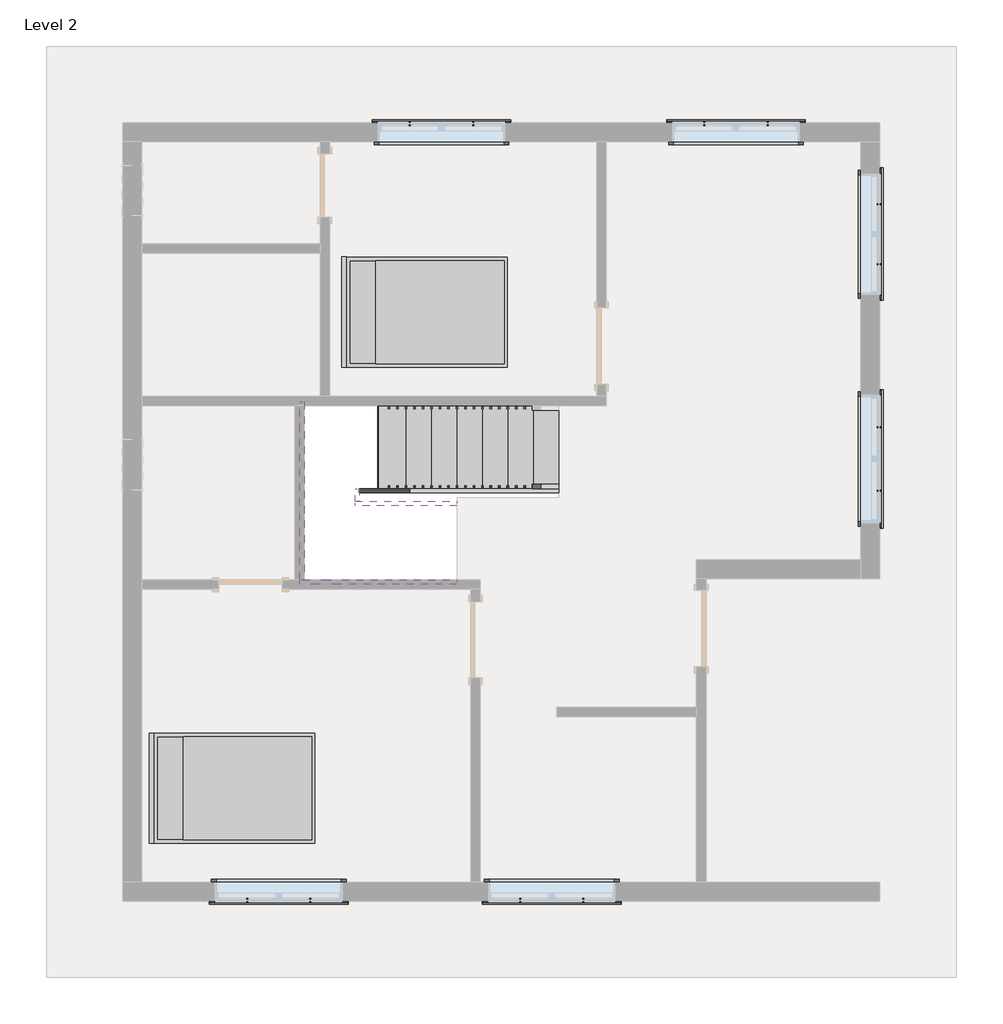
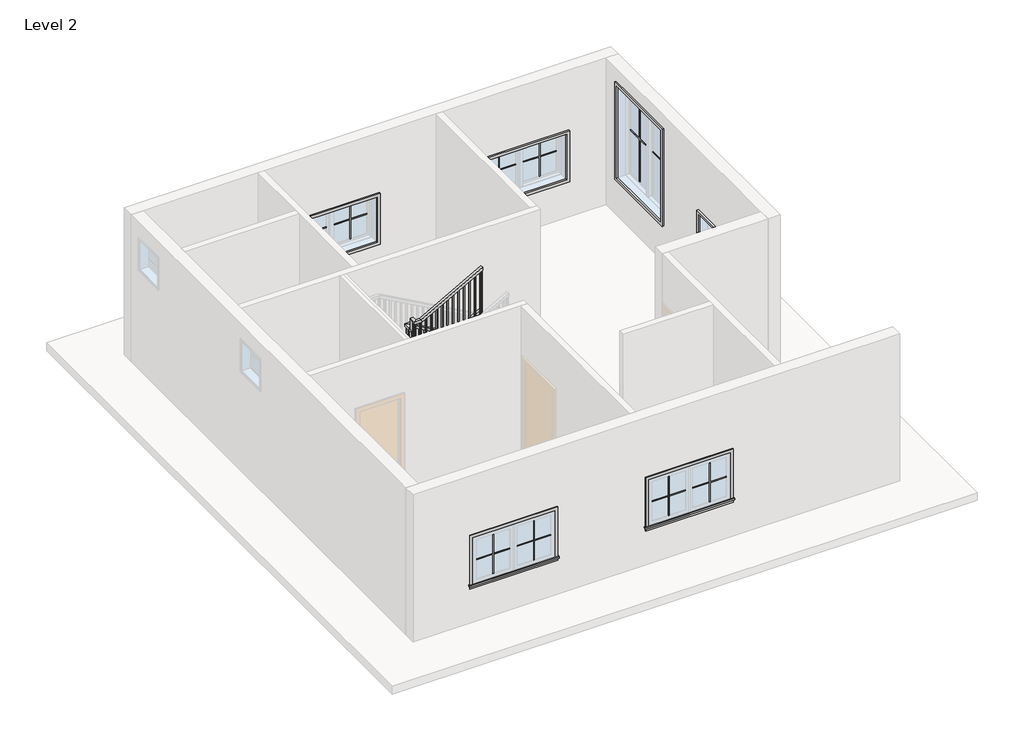
# One storey, part 2 of 2: 24 proxies, 6 members, 2 furniture elements, 1 railing, 1 stair flight.
"""IFC4 building model written with IfcOpenShell, lengths in millimetres."""

from ifc_helpers import new_model, si_unit, frame, origin, place, context, project, spatial, polyline, outline, extrude, faceted_brep, transform, mapped, element, save
from components import muntin_pattern_2x2_muntin_pattern_2x2_9352d081, muntin_pattern_2x2_muntin_pattern_2x2_5c2cbe28, muntin_pattern_2x2_muntin_pattern_2x2_bff912c5, muntin_pattern_2x2_muntin_pattern_2x2_c2194282, trim_window_exterior_flat_with_sill_979bde60, trim_window_exterior_flat_with_sill_e04b3088, trim_window_interior_flat_picture_frame_7883d11b, trim_window_interior_flat_picture_frame_2a7685fe, bed_17739_bed_17739_15c61121, stair_flight_d10e185a

model = new_model("IFC4")

# Units and contexts
model_context = context("Model", 3, world=origin())
ifc_project = project(units=[si_unit("LENGTHUNIT", "METRE", prefix="MILLI")], contexts=[model_context])

# Site, building, storey
site = spatial("IfcSite", under=ifc_project)
building = spatial("IfcBuilding", under=site)
storey = spatial("IfcBuildingStorey", under=building, Name="Level 2", Elevation=3048.0)

# Proxies
placement = place(None, origin())
muntin_pattern_2x2_muntin_pattern_2x2_shape = muntin_pattern_2x2_muntin_pattern_2x2_9352d081(model_context)
element("IfcBuildingElementProxy", 1, Name="Muntin Pattern_2x2 : Muntin Pattern_2x2", ObjectType="Muntin Pattern_2x2 : Muntin Pattern_2x2", at=placement, inside=storey, context=model_context, shape_type="MappedRepresentation", body=[
    mapped(muntin_pattern_2x2_muntin_pattern_2x2_shape, transform((-3542.9505704, -5264.0292021, 4032.25), x_axis=(-1.0, 0.0, 0.0), y_axis=(0.0, -1.0, 0.0), z_axis=(0.0, 0.0, 1.0))),
])
element("IfcBuildingElementProxy", 2, Name="Muntin Pattern_2x2 : Muntin Pattern_2x2", ObjectType="Muntin Pattern_2x2 : Muntin Pattern_2x2", at=placement, inside=storey, context=model_context, shape_type="MappedRepresentation", body=[
    mapped(muntin_pattern_2x2_muntin_pattern_2x2_shape, transform((-272.7005704, -5264.0292021, 4032.25), x_axis=(-1.0, 0.0, 0.0), y_axis=(0.0, -1.0, 0.0), z_axis=(0.0, 0.0, 1.0))),
])
element("IfcBuildingElementProxy", 3, Name="Muntin Pattern_2x2 : Muntin Pattern_2x2", ObjectType="Muntin Pattern_2x2 : Muntin Pattern_2x2", at=placement, inside=storey, context=model_context, shape_type="MappedRepresentation", body=[
    mapped(muntin_pattern_2x2_muntin_pattern_2x2_shape, transform((3269.0119296, 401.7582979, 4032.25), x_axis=(0.0, -1.0, 0.0), y_axis=(1.0, 0.0, 0.0), z_axis=(0.0, 0.0, 1.0))),
])
element("IfcBuildingElementProxy", 4, Name="Muntin Pattern_2x2 : Muntin Pattern_2x2", ObjectType="Muntin Pattern_2x2 : Muntin Pattern_2x2", at=placement, inside=storey, context=model_context, shape_type="MappedRepresentation", body=[
    mapped(muntin_pattern_2x2_muntin_pattern_2x2_shape, transform((1175.0994296, 4038.7207979, 4032.25), x_axis=(1.0, 0.0, 0.0), y_axis=(0.0, 1.0, 0.0), z_axis=(0.0, 0.0, 1.0))),
])
element("IfcBuildingElementProxy", 5, Name="Muntin Pattern_2x2 : Muntin Pattern_2x2", ObjectType="Muntin Pattern_2x2 : Muntin Pattern_2x2", at=placement, inside=storey, context=model_context, shape_type="MappedRepresentation", body=[
    mapped(muntin_pattern_2x2_muntin_pattern_2x2_shape, transform((-2352.3255704, 4038.7207979, 4032.25), x_axis=(1.0, 0.0, 0.0), y_axis=(0.0, 1.0, 0.0), z_axis=(0.0, 0.0, 1.0))),
])
muntin_pattern_2x2_muntin_pattern_2x2_2_shape = muntin_pattern_2x2_muntin_pattern_2x2_5c2cbe28(model_context)
element("IfcBuildingElementProxy", 6, Name="Muntin Pattern_2x2 : Muntin Pattern_2x2", ObjectType="Muntin Pattern_2x2 : Muntin Pattern_2x2", at=placement, inside=storey, context=model_context, shape_type="MappedRepresentation", body=[
    mapped(muntin_pattern_2x2_muntin_pattern_2x2_2_shape, transform((-4301.7755704, -5264.0292021, 4032.25), x_axis=(1.0, 0.0, 0.0), y_axis=(0.0, 1.0, 0.0), z_axis=(0.0, 0.0, 1.0))),
])
element("IfcBuildingElementProxy", 7, Name="Muntin Pattern_2x2 : Muntin Pattern_2x2", ObjectType="Muntin Pattern_2x2 : Muntin Pattern_2x2", at=placement, inside=storey, context=model_context, shape_type="MappedRepresentation", body=[
    mapped(muntin_pattern_2x2_muntin_pattern_2x2_2_shape, transform((-1031.5255704, -5264.0292021, 4032.25), x_axis=(1.0, 0.0, 0.0), y_axis=(0.0, 1.0, 0.0), z_axis=(0.0, 0.0, 1.0))),
])
element("IfcBuildingElementProxy", 8, Name="Muntin Pattern_2x2 : Muntin Pattern_2x2", ObjectType="Muntin Pattern_2x2 : Muntin Pattern_2x2", at=placement, inside=storey, context=model_context, shape_type="MappedRepresentation", body=[
    mapped(muntin_pattern_2x2_muntin_pattern_2x2_2_shape, transform((3269.0119296, -357.0667021, 4032.25), x_axis=(0.0, 1.0, 0.0), y_axis=(-1.0, 0.0, 0.0), z_axis=(0.0, 0.0, 1.0))),
])
element("IfcBuildingElementProxy", 9, Name="Muntin Pattern_2x2 : Muntin Pattern_2x2", ObjectType="Muntin Pattern_2x2 : Muntin Pattern_2x2", at=placement, inside=storey, context=model_context, shape_type="MappedRepresentation", body=[
    mapped(muntin_pattern_2x2_muntin_pattern_2x2_2_shape, transform((1933.9244296, 4038.7207979, 4032.25), x_axis=(-1.0, 0.0, 0.0), y_axis=(0.0, -1.0, 0.0), z_axis=(0.0, 0.0, 1.0))),
])
element("IfcBuildingElementProxy", 10, Name="Muntin Pattern_2x2 : Muntin Pattern_2x2", ObjectType="Muntin Pattern_2x2 : Muntin Pattern_2x2", at=placement, inside=storey, context=model_context, shape_type="MappedRepresentation", body=[
    mapped(muntin_pattern_2x2_muntin_pattern_2x2_2_shape, transform((-1593.5005704, 4038.7207979, 4032.25), x_axis=(-1.0, 0.0, 0.0), y_axis=(0.0, -1.0, 0.0), z_axis=(0.0, 0.0, 1.0))),
])
muntin_pattern_2x2_muntin_pattern_2x2_3_shape = muntin_pattern_2x2_muntin_pattern_2x2_bff912c5(model_context)
element("IfcBuildingElementProxy", 11, Name="Muntin Pattern_2x2 : Muntin Pattern_2x2", ObjectType="Muntin Pattern_2x2 : Muntin Pattern_2x2", at=placement, inside=storey, context=model_context, shape_type="MappedRepresentation", body=[
    mapped(muntin_pattern_2x2_muntin_pattern_2x2_3_shape, transform((3269.0119296, 3075.1082979, 4032.25), x_axis=(0.0, -1.0, 0.0), y_axis=(1.0, 0.0, 0.0), z_axis=(0.0, 0.0, 1.0))),
])
muntin_pattern_2x2_muntin_pattern_2x2_4_shape = muntin_pattern_2x2_muntin_pattern_2x2_c2194282(model_context)
element("IfcBuildingElementProxy", 12, Name="Muntin Pattern_2x2 : Muntin Pattern_2x2", ObjectType="Muntin Pattern_2x2 : Muntin Pattern_2x2", at=placement, inside=storey, context=model_context, shape_type="MappedRepresentation", body=[
    mapped(muntin_pattern_2x2_muntin_pattern_2x2_4_shape, transform((3269.0119296, 2354.3832979, 4032.25), x_axis=(0.0, 1.0, 0.0), y_axis=(-1.0, 0.0, 0.0), z_axis=(0.0, 0.0, 1.0))),
])
trim_window_exterior_flat_with_sill_shape = trim_window_exterior_flat_with_sill_979bde60(model_context)
element("IfcBuildingElementProxy", 13, Name="Trim-Window-Exterior-Flat : with Sill", ObjectType="Trim-Window-Exterior-Flat : with Sill", at=placement, inside=storey, context=model_context, shape_type="MappedRepresentation", body=[
    mapped(trim_window_exterior_flat_with_sill_shape, transform((-3922.3630704, -5273.5542021, 4876.8), x_axis=(1.0, 0.0, 0.0), y_axis=(0.0, 0.0, 1.0), z_axis=(0.0, -1.0, 0.0))),
])
element("IfcBuildingElementProxy", 14, Name="Trim-Window-Exterior-Flat : with Sill", ObjectType="Trim-Window-Exterior-Flat : with Sill", at=placement, inside=storey, context=model_context, shape_type="MappedRepresentation", body=[
    mapped(trim_window_exterior_flat_with_sill_shape, transform((-652.1130704, -5273.5542021, 4876.8), x_axis=(1.0, 0.0, 0.0), y_axis=(0.0, 0.0, 1.0), z_axis=(0.0, -1.0, 0.0))),
])
element("IfcBuildingElementProxy", 15, Name="Trim-Window-Exterior-Flat : with Sill", ObjectType="Trim-Window-Exterior-Flat : with Sill", at=placement, inside=storey, context=model_context, shape_type="MappedRepresentation", body=[
    mapped(trim_window_exterior_flat_with_sill_shape, transform((3278.5369296, 22.3457979, 4876.8), x_axis=(0.0, 1.0, 0.0), y_axis=(0.0, 0.0, 1.0), z_axis=(1.0, 0.0, 0.0))),
])
element("IfcBuildingElementProxy", 16, Name="Trim-Window-Exterior-Flat : with Sill", ObjectType="Trim-Window-Exterior-Flat : with Sill", at=placement, inside=storey, context=model_context, shape_type="MappedRepresentation", body=[
    mapped(trim_window_exterior_flat_with_sill_shape, transform((1554.5119296, 4048.2457979, 4876.8), x_axis=(-1.0, 0.0, 0.0), y_axis=(0.0, 0.0, 1.0), z_axis=(0.0, 1.0, 0.0))),
])
element("IfcBuildingElementProxy", 17, Name="Trim-Window-Exterior-Flat : with Sill", ObjectType="Trim-Window-Exterior-Flat : with Sill", at=placement, inside=storey, context=model_context, shape_type="MappedRepresentation", body=[
    mapped(trim_window_exterior_flat_with_sill_shape, transform((-1972.9130704, 4048.2457979, 4876.8), x_axis=(-1.0, 0.0, 0.0), y_axis=(0.0, 0.0, 1.0), z_axis=(0.0, 1.0, 0.0))),
])
trim_window_exterior_flat_with_sill_2_shape = trim_window_exterior_flat_with_sill_e04b3088(model_context)
element("IfcBuildingElementProxy", 18, Name="Trim-Window-Exterior-Flat : with Sill", ObjectType="Trim-Window-Exterior-Flat : with Sill", at=placement, inside=storey, context=model_context, shape_type="MappedRepresentation", body=[
    mapped(trim_window_exterior_flat_with_sill_2_shape, transform((3278.5369296, 2714.7457979, 5791.2), x_axis=(0.0, 1.0, 0.0), y_axis=(0.0, 0.0, 1.0), z_axis=(1.0, 0.0, 0.0))),
])
trim_window_interior_flat_picture_frame_shape = trim_window_interior_flat_picture_frame_7883d11b(model_context)
element("IfcBuildingElementProxy", 19, Name="Trim-Window-Interior-Flat : Picture Frame", ObjectType="Trim-Window-Interior-Flat : Picture Frame", at=placement, inside=storey, context=model_context, shape_type="MappedRepresentation", body=[
    mapped(trim_window_interior_flat_picture_frame_shape, transform((-3922.3630704, -5044.9542021, 4876.8), x_axis=(-1.0, 0.0, 0.0), y_axis=(0.0, 0.0, 1.0), z_axis=(0.0, 1.0, 0.0))),
])
element("IfcBuildingElementProxy", 20, Name="Trim-Window-Interior-Flat : Picture Frame", ObjectType="Trim-Window-Interior-Flat : Picture Frame", at=placement, inside=storey, context=model_context, shape_type="MappedRepresentation", body=[
    mapped(trim_window_interior_flat_picture_frame_shape, transform((-652.1130704, -5044.9542021, 4876.8), x_axis=(-1.0, 0.0, 0.0), y_axis=(0.0, 0.0, 1.0), z_axis=(0.0, 1.0, 0.0))),
])
element("IfcBuildingElementProxy", 21, Name="Trim-Window-Interior-Flat : Picture Frame", ObjectType="Trim-Window-Interior-Flat : Picture Frame", at=placement, inside=storey, context=model_context, shape_type="MappedRepresentation", body=[
    mapped(trim_window_interior_flat_picture_frame_shape, transform((3049.9369296, 22.3457979, 4876.8), x_axis=(0.0, -1.0, 0.0), y_axis=(0.0, 0.0, 1.0), z_axis=(-1.0, 0.0, 0.0))),
])
element("IfcBuildingElementProxy", 22, Name="Trim-Window-Interior-Flat : Picture Frame", ObjectType="Trim-Window-Interior-Flat : Picture Frame", at=placement, inside=storey, context=model_context, shape_type="MappedRepresentation", body=[
    mapped(trim_window_interior_flat_picture_frame_shape, transform((1554.5119296, 3819.6457979, 4876.8), x_axis=(1.0, 0.0, 0.0), y_axis=(0.0, 0.0, 1.0), z_axis=(0.0, -1.0, 0.0))),
])
element("IfcBuildingElementProxy", 23, Name="Trim-Window-Interior-Flat : Picture Frame", ObjectType="Trim-Window-Interior-Flat : Picture Frame", at=placement, inside=storey, context=model_context, shape_type="MappedRepresentation", body=[
    mapped(trim_window_interior_flat_picture_frame_shape, transform((-1972.9130704, 3819.6457979, 4876.8), x_axis=(1.0, 0.0, 0.0), y_axis=(0.0, 0.0, 1.0), z_axis=(0.0, -1.0, 0.0))),
])
trim_window_interior_flat_picture_frame_2_shape = trim_window_interior_flat_picture_frame_2a7685fe(model_context)
element("IfcBuildingElementProxy", 24, Name="Trim-Window-Interior-Flat : Picture Frame", ObjectType="Trim-Window-Interior-Flat : Picture Frame", at=placement, inside=storey, context=model_context, shape_type="MappedRepresentation", body=[
    mapped(trim_window_interior_flat_picture_frame_2_shape, transform((3049.9369296, 2714.7457979, 5791.2), x_axis=(0.0, -1.0, 0.0), y_axis=(0.0, 0.0, 1.0), z_axis=(-1.0, 0.0, 0.0))),
])

# Furniture
bed_17739_bed_17739_shape = bed_17739_bed_17739_15c61121(model_context)
element("IfcFurniture", 25, ObjectType="Bed_17739 : Bed_17739", at=placement, inside=storey, context=model_context, shape_type="MappedRepresentation", body=[
    mapped(bed_17739_bed_17739_shape, transform((-4455.7630704, -3920.5467683, 3048.0), x_axis=(0.0, 1.0, 0.0), y_axis=(-1.0, 0.0, 0.0), z_axis=(0.0, 0.0, 1.0))),
])
element("IfcFurniture", 26, ObjectType="Bed_17739 : Bed_17739", at=placement, inside=storey, context=model_context, shape_type="MappedRepresentation", body=[
    mapped(bed_17739_bed_17739_shape, transform((-2150.7130704, 1781.2957979, 3048.0), x_axis=(0.0, 1.0, 0.0), y_axis=(-1.0, 0.0, 0.0), z_axis=(0.0, 0.0, 1.0))),
])

# Members
element("IfcMember", 27, ObjectType="Stringer - 2\" Width", at=placement, inside=storey, context=model_context, shape_type="SweptSolid", body=[
    extrude(outline(polyline([(3048.0, -569.5630704), (3255.5983948, -569.5630704), (4582.0428392, -2957.1630704), (4233.3641651, -2957.1630704), (3048.0, -823.5075732), (3048.0, -569.5630704)])), frame((0.0, -384.0542021, 0.0), z_axis=(0.0, 1.0, 0.0), x_axis=(0.0, 0.0, 1.0)), (0.0, 0.0, 1.0), 50.8),
])
element("IfcMember", 28, ObjectType="Stringer - 2\" Width", at=placement, inside=storey, context=model_context, shape_type="SweptSolid", body=[
    extrude(outline(polyline([(-3007.9630704, -333.2542021), (-2957.1630704, -333.2542021), (-2957.1630704, -485.6542021), (-3007.9630704, -485.6542021), (-3007.9630704, -333.2542021)])), frame((0.0, 0.0, 4343.4), z_axis=(0.0, 0.0, 1.0), x_axis=(1.0, 0.0, 0.0)), (0.0, 0.0, 1.0), 304.8),
])
element("IfcMember", 29, ObjectType="Stringer - 2\" Width", at=placement, inside=storey, context=model_context, shape_type="SweptSolid", body=[
    extrude(outline(polyline([(4779.5983948, -3007.9630704), (4430.9197207, -3007.9630704), (5108.253054, -1788.7630704), (5456.9317281, -1788.7630704), (4779.5983948, -3007.9630704)])), frame((0.0, -536.4542021, 0.0), z_axis=(0.0, 1.0, 0.0), x_axis=(0.0, 0.0, 1.0)), (0.0, 0.0, 1.0), 50.8),
])
element("IfcMember", 30, ObjectType="Stringer - 2\" Width", at=placement, inside=storey, context=model_context, shape_type="SweptSolid", body=[
    extrude(outline(polyline([(3048.0, -569.5630704), (3255.5983948, -569.5630704), (4648.2, -3076.2459598), (4648.2, -3617.5630704), (4600.253054, -3617.5630704), (3048.0, -823.5075732), (3048.0, -569.5630704)])), frame((0.0, 657.3457979, 0.0), z_axis=(0.0, 1.0, 0.0), x_axis=(0.0, 0.0, 1.0)), (0.0, 0.0, 1.0), 50.8),
])
element("IfcMember", 31, ObjectType="Stringer - 2\" Width", at=placement, inside=storey, context=model_context, shape_type="SweptSolid", body=[
    extrude(outline(polyline([(-3668.3630704, 708.1457979), (-3617.5630704, 708.1457979), (-3617.5630704, -1425.4542021), (-3668.3630704, -1425.4542021), (-3668.3630704, 708.1457979)])), frame((0.0, 0.0, 4343.4), z_axis=(0.0, 0.0, 1.0), x_axis=(1.0, 0.0, 0.0)), (0.0, 0.0, 1.0), 304.8),
])
element("IfcMember", 32, ObjectType="Stringer - 2\" Width", at=placement, inside=storey, context=model_context, shape_type="SweptSolid", body=[
    extrude(outline(polyline([(4412.7095059, -3668.3630704), (4343.4, -3668.3630704), (4343.4, -3165.4985677), (5108.253054, -1788.7630704), (5456.9317281, -1788.7630704), (4412.7095059, -3668.3630704)])), frame((0.0, -1476.2542021, 0.0), z_axis=(0.0, 1.0, 0.0), x_axis=(0.0, 0.0, 1.0)), (0.0, 0.0, 1.0), 50.8),
])

# Railing
element("IfcRailing", 33, ObjectType="Handrail - Rectangular", at=placement, inside=storey, context=model_context, shape_type="SolidModel", body=[
    faceted_brep([(-569.5630704, -333.2542021, 4131.7333333), (-569.5630704, -333.2542021, 4073.620221), (-569.5630704, -282.4542021, 4073.620221), (-569.5630704, -282.4542021, 4131.7333333), (-2931.7630704, -333.2542021, 5444.0666667), (-2982.5630704, -333.2542021, 5414.1757765), (-2982.5630704, -282.4542021, 5414.1757765), (-2931.7630704, -282.4542021, 5444.0666667), (-2931.7630704, -333.2542021, 5486.4), (-2982.5630704, -333.2542021, 5435.6), (-2982.5630704, -282.4542021, 5435.6), (-2931.7630704, -282.4542021, 5486.4), (-3007.9630704, -333.2542021, 5486.4), (-3007.9630704, -333.2542021, 5435.6), (-3058.7630704, -282.4542021, 5435.6), (-3058.7630704, -282.4542021, 5486.4), (-3007.9630704, -409.4542021, 5486.4), (-3007.9630704, -409.4542021, 5435.6), (-3058.7630704, -409.4542021, 5435.6), (-3058.7630704, -409.4542021, 5486.4), (-3007.9630704, -460.2542021, 5486.4), (-3007.9630704, -511.0542021, 5435.6), (-3058.7630704, -511.0542021, 5435.6), (-3058.7630704, -460.2542021, 5486.4), (-3007.9630704, -460.2542021, 5698.0666667), (-3007.9630704, -511.0542021, 5647.2666667), (-3058.7630704, -511.0542021, 5647.2666667), (-3058.7630704, -460.2542021, 5698.0666667), (-3007.9630704, -536.4542021, 5698.0666667), (-3007.9630704, -536.4542021, 5647.2666667), (-3058.7630704, -587.2542021, 5647.2666667), (-3058.7630704, -587.2542021, 5698.0666667), (-2931.7630704, -536.4542021, 5698.0666667), (-2918.5994682, -536.4542021, 5647.2666667), (-2918.5994682, -587.2542021, 5647.2666667), (-2931.7630704, -587.2542021, 5698.0666667), (-1788.7630704, -536.4542021, 6333.0666667), (-1788.7630704, -587.2542021, 6333.0666667), (-1788.7630704, -587.2542021, 6274.9535543), (-1788.7630704, -536.4542021, 6274.9535543)], [[[0, 1, 2, 3]], [[1, 0, 4, 5]], [[2, 1, 5, 6]], [[3, 2, 6, 7]], [[0, 3, 7, 4]], [[5, 4, 8, 9]], [[6, 5, 9, 10]], [[7, 6, 10, 11]], [[4, 7, 11, 8]], [[9, 8, 12, 13]], [[10, 9, 13, 14]], [[11, 10, 14, 15]], [[8, 11, 15, 12]], [[13, 12, 16, 17]], [[14, 13, 17, 18]], [[15, 14, 18, 19]], [[12, 15, 19, 16]], [[17, 16, 20, 21]], [[18, 17, 21, 22]], [[19, 18, 22, 23]], [[16, 19, 23, 20]], [[21, 20, 24, 25]], [[22, 21, 25, 26]], [[23, 22, 26, 27]], [[20, 23, 27, 24]], [[25, 24, 28, 29]], [[26, 25, 29, 30]], [[27, 26, 30, 31]], [[24, 27, 31, 28]], [[29, 28, 32, 33]], [[30, 29, 33, 34]], [[31, 30, 34, 35]], [[28, 31, 35, 32]], [[36, 37, 38, 39]], [[33, 32, 36, 39]], [[34, 33, 39, 38]], [[35, 34, 38, 37]], [[32, 35, 37, 36]]]),
    extrude(outline(polyline([(6255.5507765, -1823.6880704), (5249.3333333, -1823.6880704), (5249.3333333, -1804.6380704), (6266.1341099, -1804.6380704), (6255.5507765, -1823.6880704)])), frame((0.0, -571.3792021, 0.0), z_axis=(0.0, 1.0, 0.0), x_axis=(0.0, 0.0, 1.0)), (0.0, 0.0, 1.0), 19.05),
    extrude(outline(polyline([(6199.1063321, -1925.2880704), (5249.3333333, -1925.2880704), (5249.3333333, -1906.2380704), (6209.6896654, -1906.2380704), (6199.1063321, -1925.2880704)])), frame((0.0, -571.3792021, 0.0), z_axis=(0.0, 1.0, 0.0), x_axis=(0.0, 0.0, 1.0)), (0.0, 0.0, 1.0), 19.05),
    extrude(outline(polyline([(6142.6618876, -2026.8880704), (5249.3333333, -2026.8880704), (5249.3333333, -2007.8380704), (6153.245221, -2007.8380704), (6142.6618876, -2026.8880704)])), frame((0.0, -571.3792021, 0.0), z_axis=(0.0, 1.0, 0.0), x_axis=(0.0, 0.0, 1.0)), (0.0, 0.0, 1.0), 19.05),
    extrude(outline(polyline([(6086.2174432, -2128.4880704), (5080.0, -2128.4880704), (5080.0, -2109.4380704), (6096.8007765, -2109.4380704), (6086.2174432, -2128.4880704)])), frame((0.0, -571.3792021, 0.0), z_axis=(0.0, 1.0, 0.0), x_axis=(0.0, 0.0, 1.0)), (0.0, 0.0, 1.0), 19.05),
    extrude(outline(polyline([(6029.7729988, -2230.0880704), (5080.0, -2230.0880704), (5080.0, -2211.0380704), (6040.3563321, -2211.0380704), (6029.7729988, -2230.0880704)])), frame((0.0, -571.3792021, 0.0), z_axis=(0.0, 1.0, 0.0), x_axis=(0.0, 0.0, 1.0)), (0.0, 0.0, 1.0), 19.05),
    extrude(outline(polyline([(5973.3285543, -2331.6880704), (5080.0, -2331.6880704), (5080.0, -2312.6380704), (5983.9118876, -2312.6380704), (5973.3285543, -2331.6880704)])), frame((0.0, -571.3792021, 0.0), z_axis=(0.0, 1.0, 0.0), x_axis=(0.0, 0.0, 1.0)), (0.0, 0.0, 1.0), 19.05),
    extrude(outline(polyline([(5916.8841099, -2433.2880704), (4910.6666667, -2433.2880704), (4910.6666667, -2414.2380704), (5927.4674432, -2414.2380704), (5916.8841099, -2433.2880704)])), frame((0.0, -571.3792021, 0.0), z_axis=(0.0, 1.0, 0.0), x_axis=(0.0, 0.0, 1.0)), (0.0, 0.0, 1.0), 19.05),
    extrude(outline(polyline([(5860.4396654, -2534.8880704), (4910.6666667, -2534.8880704), (4910.6666667, -2515.8380704), (5871.0229988, -2515.8380704), (5860.4396654, -2534.8880704)])), frame((0.0, -571.3792021, 0.0), z_axis=(0.0, 1.0, 0.0), x_axis=(0.0, 0.0, 1.0)), (0.0, 0.0, 1.0), 19.05),
    extrude(outline(polyline([(5803.995221, -2636.4880704), (4910.6666667, -2636.4880704), (4910.6666667, -2617.4380704), (5814.5785543, -2617.4380704), (5803.995221, -2636.4880704)])), frame((0.0, -571.3792021, 0.0), z_axis=(0.0, 1.0, 0.0), x_axis=(0.0, 0.0, 1.0)), (0.0, 0.0, 1.0), 19.05),
    extrude(outline(polyline([(5747.5507765, -2738.0880704), (4741.3333333, -2738.0880704), (4741.3333333, -2719.0380704), (5758.1341099, -2719.0380704), (5747.5507765, -2738.0880704)])), frame((0.0, -571.3792021, 0.0), z_axis=(0.0, 1.0, 0.0), x_axis=(0.0, 0.0, 1.0)), (0.0, 0.0, 1.0), 19.05),
    extrude(outline(polyline([(5691.1063321, -2839.6880704), (4741.3333333, -2839.6880704), (4741.3333333, -2820.6380704), (5701.6896654, -2820.6380704), (5691.1063321, -2839.6880704)])), frame((0.0, -571.3792021, 0.0), z_axis=(0.0, 1.0, 0.0), x_axis=(0.0, 0.0, 1.0)), (0.0, 0.0, 1.0), 19.05),
    extrude(outline(polyline([(5634.6618876, -2941.2880704), (4741.3333333, -2941.2880704), (4741.3333333, -2922.2380704), (5645.245221, -2922.2380704), (5634.6618876, -2941.2880704)])), frame((0.0, -571.3792021, 0.0), z_axis=(0.0, 1.0, 0.0), x_axis=(0.0, 0.0, 1.0)), (0.0, 0.0, 1.0), 19.05),
    extrude(outline(polyline([(-3023.8380704, -501.5292021), (-3023.8380704, -520.5792021), (-3042.8880704, -520.5792021), (-3042.8880704, -501.5292021), (-3023.8380704, -501.5292021)])), frame((0.0, 0.0, 4572.0), z_axis=(0.0, 0.0, 1.0), x_axis=(1.0, 0.0, 0.0)), (0.0, 0.0, 1.0), 1075.2666667),
    extrude(outline(polyline([(-3023.8380704, -399.9292021), (-3023.8380704, -418.9792021), (-3042.8880704, -418.9792021), (-3042.8880704, -399.9292021), (-3023.8380704, -399.9292021)])), frame((0.0, 0.0, 4572.0), z_axis=(0.0, 0.0, 1.0), x_axis=(1.0, 0.0, 0.0)), (0.0, 0.0, 1.0), 863.6),
    extrude(outline(polyline([(-2998.4380704, -317.3792021), (-3017.4880704, -317.3792021), (-3017.4880704, -298.3292021), (-2998.4380704, -298.3292021), (-2998.4380704, -317.3792021)])), frame((0.0, 0.0, 4572.0), z_axis=(0.0, 0.0, 1.0), x_axis=(1.0, 0.0, 0.0)), (0.0, 0.0, 1.0), 863.6),
    extrude(outline(polyline([(5377.1341099, -2915.8880704), (4402.6666667, -2915.8880704), (4402.6666667, -2896.8380704), (5366.5507765, -2896.8380704), (5377.1341099, -2915.8880704)])), frame((0.0, -317.3792021, 0.0), z_axis=(0.0, 1.0, 0.0), x_axis=(0.0, 0.0, 1.0)), (0.0, 0.0, 1.0), 19.05),
    extrude(outline(polyline([(5320.6896654, -2814.2880704), (4402.6666667, -2814.2880704), (4402.6666667, -2795.2380704), (5310.1063321, -2795.2380704), (5320.6896654, -2814.2880704)])), frame((0.0, -317.3792021, 0.0), z_axis=(0.0, 1.0, 0.0), x_axis=(0.0, 0.0, 1.0)), (0.0, 0.0, 1.0), 19.05),
    extrude(outline(polyline([(5264.245221, -2712.6880704), (4402.6666667, -2712.6880704), (4402.6666667, -2693.6380704), (5253.6618876, -2693.6380704), (5264.245221, -2712.6880704)])), frame((0.0, -317.3792021, 0.0), z_axis=(0.0, 1.0, 0.0), x_axis=(0.0, 0.0, 1.0)), (0.0, 0.0, 1.0), 19.05),
    extrude(outline(polyline([(5207.8007765, -2611.0880704), (4233.3333333, -2611.0880704), (4233.3333333, -2592.0380704), (5197.2174432, -2592.0380704), (5207.8007765, -2611.0880704)])), frame((0.0, -317.3792021, 0.0), z_axis=(0.0, 1.0, 0.0), x_axis=(0.0, 0.0, 1.0)), (0.0, 0.0, 1.0), 19.05),
    extrude(outline(polyline([(5151.3563321, -2509.4880704), (4233.3333333, -2509.4880704), (4233.3333333, -2490.4380704), (5140.7729988, -2490.4380704), (5151.3563321, -2509.4880704)])), frame((0.0, -317.3792021, 0.0), z_axis=(0.0, 1.0, 0.0), x_axis=(0.0, 0.0, 1.0)), (0.0, 0.0, 1.0), 19.05),
    extrude(outline(polyline([(5094.9118876, -2407.8880704), (4233.3333333, -2407.8880704), (4233.3333333, -2388.8380704), (5084.3285543, -2388.8380704), (5094.9118876, -2407.8880704)])), frame((0.0, -317.3792021, 0.0), z_axis=(0.0, 1.0, 0.0), x_axis=(0.0, 0.0, 1.0)), (0.0, 0.0, 1.0), 19.05),
    extrude(outline(polyline([(5038.4674432, -2306.2880704), (4064.0, -2306.2880704), (4064.0, -2287.2380704), (5027.8841099, -2287.2380704), (5038.4674432, -2306.2880704)])), frame((0.0, -317.3792021, 0.0), z_axis=(0.0, 1.0, 0.0), x_axis=(0.0, 0.0, 1.0)), (0.0, 0.0, 1.0), 19.05),
    extrude(outline(polyline([(4982.0229988, -2204.6880704), (4064.0, -2204.6880704), (4064.0, -2185.6380704), (4971.4396654, -2185.6380704), (4982.0229988, -2204.6880704)])), frame((0.0, -317.3792021, 0.0), z_axis=(0.0, 1.0, 0.0), x_axis=(0.0, 0.0, 1.0)), (0.0, 0.0, 1.0), 19.05),
    extrude(outline(polyline([(4925.5785543, -2103.0880704), (4064.0, -2103.0880704), (4064.0, -2084.0380704), (4914.995221, -2084.0380704), (4925.5785543, -2103.0880704)])), frame((0.0, -317.3792021, 0.0), z_axis=(0.0, 1.0, 0.0), x_axis=(0.0, 0.0, 1.0)), (0.0, 0.0, 1.0), 19.05),
    extrude(outline(polyline([(4869.1341099, -2001.4880704), (3894.6666667, -2001.4880704), (3894.6666667, -1982.4380704), (4858.5507765, -1982.4380704), (4869.1341099, -2001.4880704)])), frame((0.0, -317.3792021, 0.0), z_axis=(0.0, 1.0, 0.0), x_axis=(0.0, 0.0, 1.0)), (0.0, 0.0, 1.0), 19.05),
    extrude(outline(polyline([(4812.6896654, -1899.8880704), (3894.6666667, -1899.8880704), (3894.6666667, -1880.8380704), (4802.1063321, -1880.8380704), (4812.6896654, -1899.8880704)])), frame((0.0, -317.3792021, 0.0), z_axis=(0.0, 1.0, 0.0), x_axis=(0.0, 0.0, 1.0)), (0.0, 0.0, 1.0), 19.05),
    extrude(outline(polyline([(4756.245221, -1798.2880704), (3894.6666667, -1798.2880704), (3894.6666667, -1779.2380704), (4745.6618876, -1779.2380704), (4756.245221, -1798.2880704)])), frame((0.0, -317.3792021, 0.0), z_axis=(0.0, 1.0, 0.0), x_axis=(0.0, 0.0, 1.0)), (0.0, 0.0, 1.0), 19.05),
    extrude(outline(polyline([(4699.8007765, -1696.6880704), (3725.3333333, -1696.6880704), (3725.3333333, -1677.6380704), (4689.2174432, -1677.6380704), (4699.8007765, -1696.6880704)])), frame((0.0, -317.3792021, 0.0), z_axis=(0.0, 1.0, 0.0), x_axis=(0.0, 0.0, 1.0)), (0.0, 0.0, 1.0), 19.05),
    extrude(outline(polyline([(4643.3563321, -1595.0880704), (3725.3333333, -1595.0880704), (3725.3333333, -1576.0380704), (4632.7729988, -1576.0380704), (4643.3563321, -1595.0880704)])), frame((0.0, -317.3792021, 0.0), z_axis=(0.0, 1.0, 0.0), x_axis=(0.0, 0.0, 1.0)), (0.0, 0.0, 1.0), 19.05),
    extrude(outline(polyline([(4586.9118876, -1493.4880704), (3725.3333333, -1493.4880704), (3725.3333333, -1474.4380704), (4576.3285543, -1474.4380704), (4586.9118876, -1493.4880704)])), frame((0.0, -317.3792021, 0.0), z_axis=(0.0, 1.0, 0.0), x_axis=(0.0, 0.0, 1.0)), (0.0, 0.0, 1.0), 19.05),
    extrude(outline(polyline([(4530.4674432, -1391.8880704), (3556.0, -1391.8880704), (3556.0, -1372.8380704), (4519.8841099, -1372.8380704), (4530.4674432, -1391.8880704)])), frame((0.0, -317.3792021, 0.0), z_axis=(0.0, 1.0, 0.0), x_axis=(0.0, 0.0, 1.0)), (0.0, 0.0, 1.0), 19.05),
    extrude(outline(polyline([(4474.0229988, -1290.2880704), (3556.0, -1290.2880704), (3556.0, -1271.2380704), (4463.4396654, -1271.2380704), (4474.0229988, -1290.2880704)])), frame((0.0, -317.3792021, 0.0), z_axis=(0.0, 1.0, 0.0), x_axis=(0.0, 0.0, 1.0)), (0.0, 0.0, 1.0), 19.05),
    extrude(outline(polyline([(4417.5785543, -1188.6880704), (3556.0, -1188.6880704), (3556.0, -1169.6380704), (4406.995221, -1169.6380704), (4417.5785543, -1188.6880704)])), frame((0.0, -317.3792021, 0.0), z_axis=(0.0, 1.0, 0.0), x_axis=(0.0, 0.0, 1.0)), (0.0, 0.0, 1.0), 19.05),
    extrude(outline(polyline([(4361.1341099, -1087.0880704), (3386.6666667, -1087.0880704), (3386.6666667, -1068.0380704), (4350.5507765, -1068.0380704), (4361.1341099, -1087.0880704)])), frame((0.0, -317.3792021, 0.0), z_axis=(0.0, 1.0, 0.0), x_axis=(0.0, 0.0, 1.0)), (0.0, 0.0, 1.0), 19.05),
    extrude(outline(polyline([(4304.6896654, -985.4880704), (3386.6666667, -985.4880704), (3386.6666667, -966.4380704), (4294.1063321, -966.4380704), (4304.6896654, -985.4880704)])), frame((0.0, -317.3792021, 0.0), z_axis=(0.0, 1.0, 0.0), x_axis=(0.0, 0.0, 1.0)), (0.0, 0.0, 1.0), 19.05),
    extrude(outline(polyline([(4248.245221, -883.8880704), (3386.6666667, -883.8880704), (3386.6666667, -864.8380704), (4237.6618876, -864.8380704), (4248.245221, -883.8880704)])), frame((0.0, -317.3792021, 0.0), z_axis=(0.0, 1.0, 0.0), x_axis=(0.0, 0.0, 1.0)), (0.0, 0.0, 1.0), 19.05),
    extrude(outline(polyline([(4191.8007765, -782.2880704), (3217.3333333, -782.2880704), (3217.3333333, -763.2380704), (4181.2174432, -763.2380704), (4191.8007765, -782.2880704)])), frame((0.0, -317.3792021, 0.0), z_axis=(0.0, 1.0, 0.0), x_axis=(0.0, 0.0, 1.0)), (0.0, 0.0, 1.0), 19.05),
    extrude(outline(polyline([(4135.3563321, -680.6880704), (3217.3333333, -680.6880704), (3217.3333333, -661.6380704), (4124.7729988, -661.6380704), (4135.3563321, -680.6880704)])), frame((0.0, -317.3792021, 0.0), z_axis=(0.0, 1.0, 0.0), x_axis=(0.0, 0.0, 1.0)), (0.0, 0.0, 1.0), 19.05),
    extrude(outline(polyline([(-3023.8380704, -552.3292021), (-3023.8380704, -571.3792021), (-3042.8880704, -571.3792021), (-3042.8880704, -552.3292021), (-3023.8380704, -552.3292021)])), frame((0.0, 0.0, 4572.0), z_axis=(0.0, 0.0, 1.0), x_axis=(1.0, 0.0, 0.0)), (0.0, 0.0, 1.0), 1075.2666667),
    extrude(outline(polyline([(-3023.8380704, -317.3792021), (-3042.8880704, -317.3792021), (-3042.8880704, -298.3292021), (-3023.8380704, -298.3292021), (-3023.8380704, -317.3792021)])), frame((0.0, 0.0, 4572.0), z_axis=(0.0, 0.0, 1.0), x_axis=(1.0, 0.0, 0.0)), (0.0, 0.0, 1.0), 863.6),
    extrude(outline(polyline([(6264.370221, -1807.8130704), (5249.3333333, -1807.8130704), (5249.3333333, -1788.7630704), (6274.9535543, -1788.7630704), (6264.370221, -1807.8130704)])), frame((0.0, -571.3792021, 0.0), z_axis=(0.0, 1.0, 0.0), x_axis=(0.0, 0.0, 1.0)), (0.0, 0.0, 1.0), 19.05),
    extrude(outline(polyline([(4084.2035543, -588.6130704), (3217.3333333, -588.6130704), (3217.3333333, -569.5630704), (4073.620221, -569.5630704), (4084.2035543, -588.6130704)])), frame((0.0, -317.3792021, 0.0), z_axis=(0.0, 1.0, 0.0), x_axis=(0.0, 0.0, 1.0)), (0.0, 0.0, 1.0), 19.05),
])

# Stair flight
stair_flight_shape = stair_flight_d10e185a(model_context)
element("IfcStairFlight", 34, ObjectType="2\" Tread 1\" Nosing 1/4\" Riser", at=placement, inside=storey, context=model_context, shape_type="MappedRepresentation", body=[
    mapped(stair_flight_shape, transform((0.0, 0.0, 0.0), x_axis=(1.0, 0.0, 0.0), y_axis=(0.0, 1.0, 0.0), z_axis=(0.0, 0.0, 1.0))),
])

save(model, "model.ifc")

# Revit data of these elements
# Type "Muntin Pattern_2x2 : Muntin Pattern_2x2"
#   Width [instance default] = 4' - 0"
#   Thickness = 0' - 0 1/2"
#   Height [instance default] = 4' - 0"
#   Distance = 0' - 0 3/4"
#   Interior Material [instance default] = none
#   Exterior Material [instance default] = none
#   Default Elevation = 0
# Type "Trim-Window-Exterior-Flat : with Sill"
#   Trim Width = 0' - 2 1/4"
#   Trim Thickness_Picture Frame = 0' - 1 1/4"
#   Trim Thickness_with Sill = 0' - 0 3/4"
#   Sill Thickness = 0' - 1 1/4"
#   Opening Width [instance default] = 2' - 0"
#   Opening Height [instance default] = 3' - 0"
#   Default Elevation = 4' - 0"
#   Sill = yes
#   Picture Frame = no
#   Trim Material [instance default] = none
# Type "Trim-Window-Interior-Flat : Picture Frame"
#   Trim Thickness_Picture Frame = 0' - 1 1/4"
#   Trim Width = 0' - 2 1/4"
#   Trim Thickness_with Sill = 0' - 0 3/4"
#   Sill Thickness = 0' - 1 1/4"
#   Opening Width [instance default] = 2' - 0"
#   Opening Height [instance default] = 3' - 0"
#   Default Elevation = 4' - 0"
#   Sill = no
#   Picture Frame = yes
#   Trim Material [instance default] = none
# Type "Bed_17739 : Bed_17739"
#   Default Elevation = 0
# Type "Handrail - Rectangular"
#   Assembly Code = "C2010400"
#   built-in parameter 1008612 = 0.0416667 (stored number, unit not read)
#   built-in parameter 1008611 = 0.0416667 (stored number, unit not read)
#   built-in parameter 1008609 = 0.333333 (stored number, unit not read)
#   built-in parameter 1008604 = 0.166667 (stored number, unit not read)
#   built-in parameter 1008603 = 0.166667 (stored number, unit not read)
#   Railing Height = 3' - 0"
#   built-in parameter 1008630 = 2
#   built-in parameter 1008610 = 2
#   built-in parameter 1008618 = Baluster - Square : 3/4"
# Elements 1, 2, 3, 4, 5, 6, 7, 8, 9, 10 (IfcBuildingElementProxy, "Muntin Pattern_2x2 : Muntin Pattern_2x2")
#   Width = 2' - 0 5/8"
#   Height = 2' - 6 1/2"
#   Interior Material = Wood - Stained
#   Exterior Material = Clad - White
#   Phase Created = New Construction
#   Materials on its faces: "Clad - White", "Wood - Stained"
# Elements 11, 12 (IfcBuildingElementProxy, "Muntin Pattern_2x2 : Muntin Pattern_2x2")
#   Width = 1' - 11 1/8"
#   Height = 5' - 6 1/2"
#   Interior Material = Wood - Stained
#   Exterior Material = Clad - White
#   Phase Created = New Construction
#   Materials on its faces: "Clad - White", "Wood - Stained"
# Elements 13, 14, 15, 16, 17 (IfcBuildingElementProxy, "Trim-Window-Exterior-Flat : with Sill")
#   Opening Width = 5' - 0"
#   Opening Height = 3' - 0"
#   Trim Material = Clad - White
#   Phase Created = New Construction
#   Materials on its faces: "Clad - White"
# Element 18 (IfcBuildingElementProxy, "Trim-Window-Exterior-Flat : with Sill")
#   Opening Width = 4' - 9"
#   Opening Height = 6' - 0"
#   Trim Material = Clad - White
#   Phase Created = New Construction
#   Materials on its faces: "Clad - White"
# Elements 19, 20, 21, 22, 23 (IfcBuildingElementProxy, "Trim-Window-Interior-Flat : Picture Frame")
#   Opening Width = 5' - 0"
#   Opening Height = 3' - 0"
#   Trim Material = Wood - Stained
#   Phase Created = New Construction
#   Materials on its faces: "Wood - Stained"
# Element 24 (IfcBuildingElementProxy, "Trim-Window-Interior-Flat : Picture Frame")
#   Opening Width = 4' - 9"
#   Opening Height = 6' - 0"
#   Trim Material = Wood - Stained
#   Phase Created = New Construction
#   Materials on its faces: "Wood - Stained"
# Elements 25, 26 (IfcFurniture, "Bed_17739 : Bed_17739")
#   Phase Created = New Construction
#   Materials on its faces: "legs", "sheets", "bed frame", "Blanket"
# Elements 27, 28, 29, 30, 31, 32 (IfcMember, "Stringer - 2\" Width")
#   Phase Created = New Construction
# Element 33 (IfcRailing, "Handrail - Rectangular")
#   Phase Created = New Construction
# Element 34 (IfcStairFlight, "2\" Tread 1\" Nosing 1/4\" Riser")
#   Phase Created = New Construction
# Materials
#   "Clad - White": class "Wood", colour RGB 242 242 238, transparency 0, Cost = 0
#   "Wood - Stained": class "Wood", colour RGB 224 178 126, transparency 0, Cost = 0
#   "legs": colour RGB 90 73 37, transparency 0, Cost = 0
#   "sheets": colour RGB 200 195 176, transparency 0, Cost = 0
#   "bed frame": colour RGB 90 73 37, transparency 0, Cost = 0
#   "Blanket": class "System", colour RGB 59 0 1, transparency 0, Cost = 0
